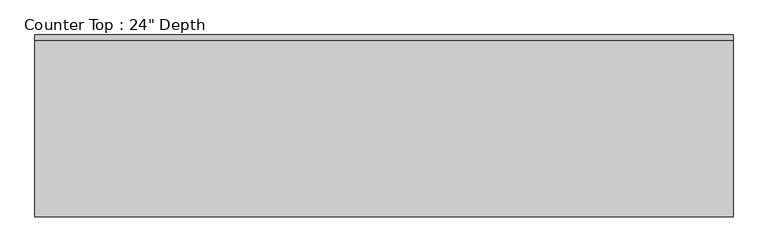
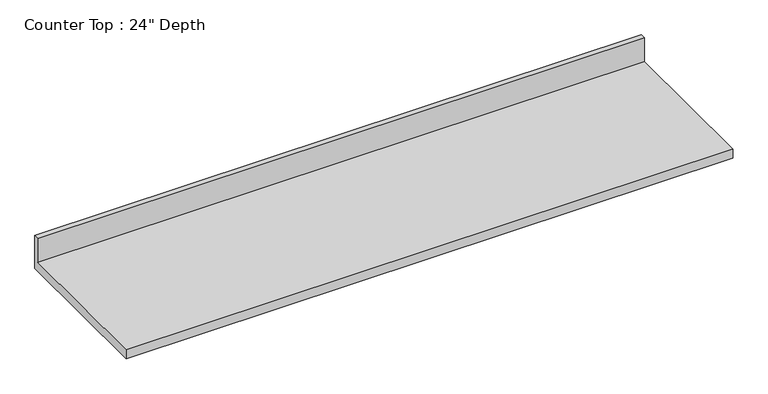
"""IFC4 building model written with IfcOpenShell, lengths in millimetres: furniture geometry."""

from ifc_helpers import new_model, si_unit, frame, origin, place, context, project, spatial, polyline, outline, extrude, source, transform, mapped, element, save


def furniture_deb1c5d1(model_context):
    return source(origin(), model_context, "Body", "SweptSolid", [
        extrude(outline(polyline([(0.0, 1016.0), (0.0, 876.3), (-635.0, 876.3), (-635.0, 914.4), (-19.05, 914.4), (-19.05, 1016.0), (0.0, 1016.0)])), frame((-1200.4622951, 0.0, 0.0), z_axis=(1.0, 0.0, 0.0), x_axis=(0.0, 1.0, 0.0)), (0.0, 0.0, 1.0), 2438.4),
    ])


if __name__ == "__main__":
    model = new_model("IFC4")
    model_context = context("Model", 3, world=origin())
    ifc_project = project(units=[si_unit("LENGTHUNIT", "METRE", prefix="MILLI")], contexts=[model_context])
    site = spatial("IfcSite", under=ifc_project)
    building = spatial("IfcBuilding", under=site)
    placement = place(None, origin())
    furniture_shape = furniture_deb1c5d1(model_context)
    element("IfcFurniture", 1, ObjectType="Counter Top : 24\" Depth", at=placement, inside=building, context=model_context, shape_type="MappedRepresentation", body=[
        mapped(furniture_shape, transform((0.0, 0.0, 0.0), x_axis=(1.0, 0.0, 0.0), y_axis=(0.0, 1.0, 0.0), z_axis=(0.0, 0.0, 1.0))),
    ])
    save(model, "model.ifc")

# Revit data of these elements
# Type "Counter Top : 24\" Depth"
#   Assembly Code = "C1030400"
#   Counter Thickness = 0.125 ft
#   Depth = 2.083333 ft
#   Height = 3 ft
#   Length [instance default] = 8 ft
#   Counter Top Material = none
#   Default Elevation = 0
# Element 1 (IfcFurniture, "Counter Top : 24\" Depth")
#   Materials on its faces: "Counter Top"
# Materials
#   "Counter Top": class "Wood", colour RGB 226 177 128, transparency 0
